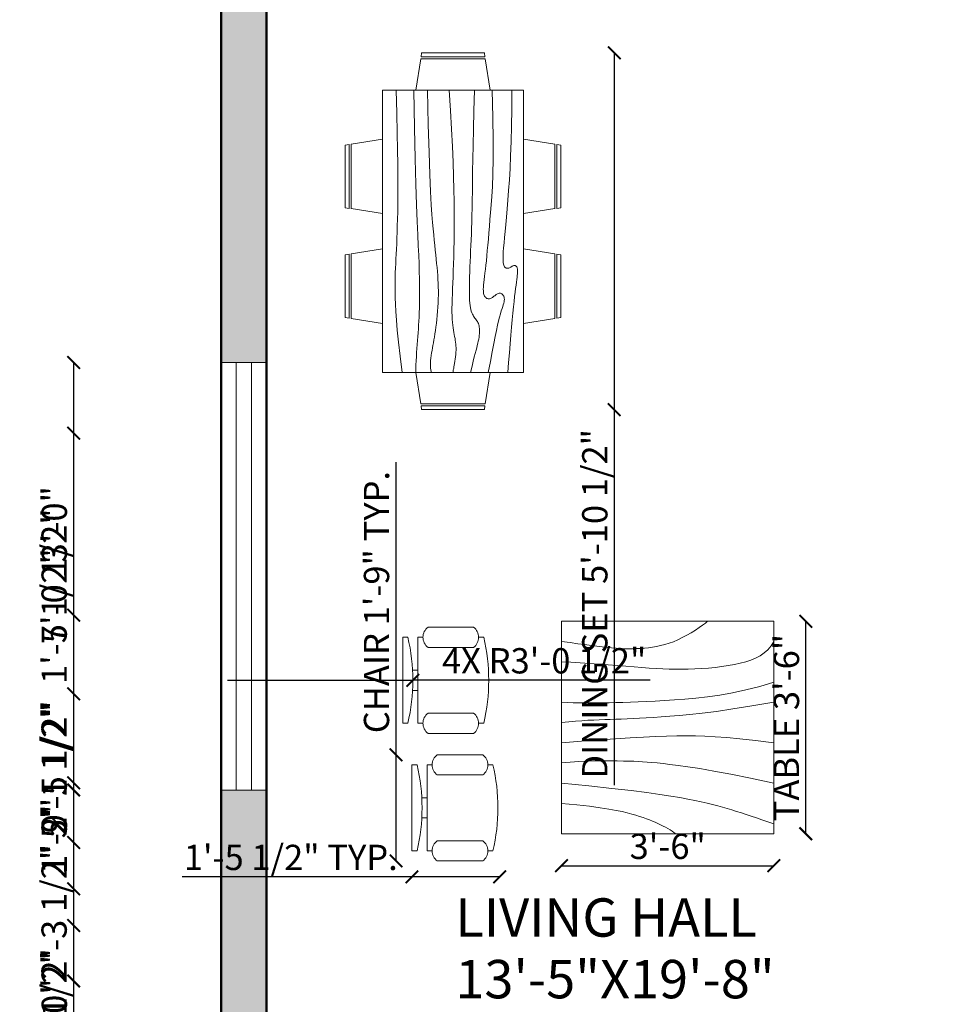
# Model space of a CAD drawing. Units: inches. Extents: x 1799 to 2247, y 1296 to 1881.
# Tile 2 of 4: x 1799 to 1983, y 1492 to 1687. Entities that reach past the tile are written whole.
import ezdxf

# ---------------------------------------------------------------- set-up
doc = ezdxf.new("R2010")
doc.units = ezdxf.units.IN
for name, color, linetype, lineweight in [('A-ANNO-DIMS', 2, 'Continuous', 18), ('A-AREA-IDEN', 7, 'Continuous', 25), ('A-FURN', 8, 'Continuous', 18), ('A-WALL', 7, 'Continuous', 50), ('window', 4, 'Continuous', 18)]:
    doc.layers.add(name, color=color, linetype=linetype, lineweight=lineweight)
doc.layers.add('A-WALL-PATT', color=18, linetype='Continuous', lineweight=13, true_color=0x000000)
doc.styles.get("Standard").update_dxf_attribs({"font": 'arial.ttf'})
doc.dimstyles.new('ISO-25', dxfattribs={"dimtxt": 5, "dimasz": 2.5, "dimexe": 1.25, "dimexo": 0.625, "dimtad": 1, "dimdec": 0, "dimlunit": 4, "dimtxsty": 'Standard', "dimblk": 'ARCHTICK', "dimcen": 2.5, "dimse1": 1, "dimse2": 1, "dimclrd": 1, "dimadec": 0, "dimazin": 0, "dimtfac": 1, "dimtdec": 0, "dimtmove": 0, "dimatfit": 3, "dimfxl": 1, "dimarcsym": 0})

# ---------------------------------------------------------------- blocks, each defined once
blk = doc.blocks.new('Dining Set - 36 x 72 in.')
for p, q in [((-22.2343, 26.00059), (-23.4847, 17.99762)), ((-22.2304, 26), (-5.7608, 26)), ((-22, 27.5), (-22.1562, 26.50042)), ((-5.8416, 26.5), (-22.1534, 26.5)), ((-22, 27.5), (-6, 27.5)), ((-5.8437, 26.49966), (-6, 27.5)), ((-4.5152, 17.99762), (-5.7655, 25.99926)), ((5.7657, 26.00059), (4.5153, 17.99762)), ((5.7696, 26), (22.2392, 26)), ((6, 27.5), (5.8438, 26.50042)), ((22.1584, 26.5), (5.8466, 26.5)), ((6, 27.5), (22, 27.5)), ((22.1563, 26.49966), (22, 27.5)), ((23.4848, 17.99762), (22.2345, 25.99926)), ((36, 18), (-36, 18)), ((-36, 18), (-36, -18)), ((36, -18), (36, 18)), ((-45.5, 8), (-44.5004, 8.15617)), ((-45.5, 8), (-45.5, -8)), ((-44.5, -8.15843), (-44.5, 8.15338)), ((-44.0006, 8.23428), (-35.9976, 9.48474)), ((-44, 8.23041), (-44, -8.23915)), ((44.0006, 8.23428), (35.9976, 9.48474)), ((44, 8.23041), (44, -8.23915)), ((44.5, -8.15843), (44.5, 8.15338)), ((45.5, 8), (44.5005, 8.15617)), ((45.5, 8), (45.5, -8)), ((-44.4997, -8.15631), (-45.5, -8)), ((-35.9976, -9.48476), (-43.9993, -8.2345)), ((35.9976, -9.48476), (43.9993, -8.2345)), ((44.4997, -8.15631), (45.5, -8)), ((-36, -18), (36, -18)), ((-22.2343, -26.0006), (-23.4847, -17.99762)), ((-4.5152, -17.99762), (-5.7655, -25.99928)), ((5.7657, -26.0006), (4.5153, -17.99762)), ((23.4848, -17.99762), (22.2345, -25.99928)), ((-22.2304, -26), (-5.7608, -26)), ((-22, -27.5), (-22.1562, -26.50044)), ((-5.8416, -26.5), (-22.1534, -26.5)), ((-22, -27.5), (-6, -27.5)), ((-5.8437, -26.49967), (-6, -27.5)), ((5.7696, -26), (22.2392, -26)), ((6, -27.5), (5.8438, -26.50044)), ((22.1584, -26.5), (5.8466, -26.5)), ((6, -27.5), (22, -27.5)), ((22.1563, -26.49967), (22, -27.5))]:
    blk.add_line(p, q)
for points in [[(-36, 15), (-31.1772, 14.97754), (-26.8079, 14.91406), (-22.8538, 14.81543), (-19.276, 14.6875), (-16.0362, 14.53613), (-13.0957, 14.36718), (-10.4159, 14.18652), (-7.9583, 14), (-5.6904, 13.81315), (-3.6035, 13.63021), (-1.6954, 13.45508), (0.0365, 13.29166), (1.5945, 13.14388), (2.9811, 13.01562), (4.1988, 12.9108), (5.25, 12.83333), (6.1393, 12.78613), (6.8802, 12.76823), (7.4883, 12.77767), (7.9792, 12.8125), (8.3685, 12.87077), (8.6719, 12.95052), (8.9049, 13.0498), (9.0833, 13.16666), (9.2205, 13.29899), (9.3216, 13.44401), (9.3895, 13.59879), (9.4271, 13.76041), (9.4373, 13.92594), (9.4232, 14.09245), (9.3875, 14.257), (9.3333, 14.41666), (9.2638, 14.56917), (9.1836, 14.71484), (9.0975, 14.85465), (9.0104, 14.98958), (8.9272, 15.1206), (8.8529, 15.2487), (8.7922, 15.37483), (8.75, 15.5), (8.7305, 15.62467), (8.7344, 15.74739), (8.7617, 15.86621), (8.8125, 15.97916), (8.8867, 16.08431), (8.9844, 16.17968), (9.1055, 16.26334), (9.25, 16.33333), (9.4189, 16.38802), (9.6172, 16.42708), (9.8506, 16.45052), (10.125, 16.45833), (10.4463, 16.45052), (10.8203, 16.42708), (11.2529, 16.38802), (11.75, 16.33333), (12.3184, 16.26318), (12.9694, 16.17838), (13.7151, 16.07991), (14.5677, 15.96875), (15.5395, 15.84586), (16.6426, 15.71224), (17.8893, 15.56884), (19.2917, 15.41666), (20.859, 15.25667), (22.5879, 15.08984), (24.4721, 14.91715), (26.5052, 14.73958), (28.6809, 14.5581), (30.9929, 14.3737), (33.4347, 14.18733), (36, 14)], [(-36, 10), (-28.9766, 10.14274), (-23.1725, 10.20442), (-18.4241, 10.19775), (-14.5677, 10.13541), (-11.4399, 10.03011), (-8.877, 9.89453), (-6.7154, 9.74137), (-4.7917, 9.58333), (-2.9698, 9.43082), (-1.2246, 9.28515), (0.4415, 9.14534), (2.026, 9.01041), (3.5266, 8.87939), (4.9408, 8.7513), (6.266, 8.62516), (7.5, 8.5), (8.6411, 8.37549), (9.6914, 8.2539), (10.6538, 8.13818), (11.5312, 8.03125), (12.3267, 7.93603), (13.043, 7.85547), (13.6831, 7.79248), (14.25, 7.75), (14.7471, 7.7303), (15.1797, 7.73307), (15.5537, 7.75732), (15.875, 7.80208), (16.1494, 7.86637), (16.3828, 7.94922), (16.5811, 8.04964), (16.75, 8.16666), (16.8944, 8.29915), (17.0143, 8.44531), (17.1089, 8.60319), (17.1771, 8.77083), (17.218, 8.94629), (17.2305, 9.1276), (17.2137, 9.31282), (17.1667, 9.5), (17.0895, 9.6875), (16.987, 9.875), (16.8649, 10.0625), (16.7292, 10.25), (16.5856, 10.4375), (16.4401, 10.625), (16.2985, 10.8125), (16.1667, 11), (16.05, 11.18733), (15.9518, 11.3737), (15.8752, 11.5581), (15.8229, 11.73958), (15.798, 11.91715), (15.8034, 12.08984), (15.842, 12.25667), (15.9167, 12.41666), (16.0295, 12.56836), (16.1784, 12.70833), (16.3605, 12.83268), (16.5729, 12.9375), (16.8127, 13.01888), (17.0768, 13.07291), (17.3625, 13.0957), (17.6667, 13.08333), (17.9894, 13.03312), (18.3418, 12.94726), (18.7382, 12.82918), (19.1927, 12.68229), (19.7195, 12.51001), (20.3327, 12.31575), (21.0465, 12.10294), (21.875, 11.875), (22.8357, 11.63354), (23.959, 11.37304), (25.2786, 11.08618), (26.8282, 10.76562), (28.6414, 10.40405), (30.752, 9.99414), (33.1936, 9.52856), (36, 9)], [(-36, 5.5), (-30.7157, 5.3348), (-26.069, 5.20963), (-21.9946, 5.11767), (-18.4271, 5.05208), (-15.3009, 5.00602), (-12.5508, 4.97265), (-10.1112, 4.94515), (-7.9167, 4.91666), (-5.909, 4.88167), (-4.0586, 4.83984), (-2.3429, 4.79215), (-0.7396, 4.73958), (0.7739, 4.6831), (2.22, 4.6237), (3.6213, 4.56233), (5, 4.5), (6.373, 4.43782), (7.7344, 4.3776), (9.0723, 4.32129), (10.375, 4.27083), (11.6309, 4.22819), (12.8281, 4.19531), (13.9551, 4.17415), (15, 4.16666), (15.954, 4.17448), (16.819, 4.19791), (17.6001, 4.23698), (18.3021, 4.29166), (18.9299, 4.36198), (19.4883, 4.44791), (19.9823, 4.54948), (20.4167, 4.66666), (20.7969, 4.79899), (21.1302, 4.94401), (21.4245, 5.09879), (21.6875, 5.26041), (21.9271, 5.42594), (22.1511, 5.59245), (22.3672, 5.757), (22.5834, 5.91666), (22.8065, 6.06868), (23.0404, 6.21093), (23.2879, 6.34147), (23.5521, 6.45833), (23.8358, 6.55957), (24.142, 6.64323), (24.4735, 6.70735), (24.8334, 6.75), (25.2235, 6.76969), (25.642, 6.76692), (26.0858, 6.74267), (26.5521, 6.69791), (27.0379, 6.63362), (27.5404, 6.55078), (28.0565, 6.45036), (28.5834, 6.33333), (29.1242, 6.19987), (29.7071, 6.04687), (30.3661, 5.87044), (31.1354, 5.66666), (32.0493, 5.43164), (33.142, 5.16146), (34.4475, 4.85221), (36, 4.5)], [(-36, -1), (-30.7915, -0.6591), (-26.0195, -0.38216), (-21.6519, -0.16284), (-17.6563, 0.00521), (-14.0005, 0.12833), (-10.6523, 0.21289), (-7.5796, 0.26522), (-4.75, 0.29166), (-2.134, 0.29793), (0.2878, 0.28711), (2.5317, 0.26163), (4.6146, 0.22396), (6.5529, 0.17651), (8.3633, 0.12174), (10.0623, 0.06209), (11.6667, 0), (13.1899, -0.06201), (14.6341, -0.1211), (15.9982, -0.17432), (17.2813, -0.21875), (18.4823, -0.25147), (19.6003, -0.26953), (20.6343, -0.27002), (21.5834, -0.25), (22.4481, -0.20768), (23.2357, -0.14584), (23.9549, -0.06836), (24.6146, 0.02083), (25.2235, 0.11784), (25.7904, 0.21875), (26.3241, 0.31966), (26.8334, 0.41666), (27.3265, 0.50618), (27.8099, 0.58593), (28.2894, 0.65397), (28.7709, 0.70833), (29.2601, 0.74707), (29.763, 0.76823), (30.2855, 0.76985), (30.8334, 0.75), (31.4088, 0.70784), (31.9994, 0.64713), (32.589, 0.57275), (33.1615, 0.48958), (33.7008, 0.4025), (34.1908, 0.3164), (34.6153, 0.23616), (34.9584, 0.16666), (35.2099, 0.11165), (35.3848, 0.07031), (35.504, 0.04069), (35.5886, 0.02083), (35.6594, 0.00879), (35.7377, 0.0026), (35.8442, 0.00032), (36, 0)], [(-36, -6.5), (-27.1843, -6.31267), (-20.084, -6.1263), (-14.469, -5.9419), (-10.1094, -5.76042), (-6.7752, -5.58285), (-4.2363, -5.41016), (-2.2629, -5.24333), (-0.625, -5.08334), (0.8708, -4.93099), (2.2715, -4.78646), (3.5872, -4.64974), (4.8281, -4.52084), (6.0046, -4.39974), (7.127, -4.28646), (8.2053, -4.18099), (9.25, -4.08334), (10.2705, -3.99382), (11.2734, -3.91407), (12.2647, -3.84603), (13.25, -3.79167), (14.2354, -3.75293), (15.2266, -3.73177), (16.2295, -3.73015), (17.25, -3.75), (18.2912, -3.79248), (19.3451, -3.85547), (20.4009, -3.93604), (21.4479, -4.03125), (22.4754, -4.13819), (23.4727, -4.25391), (24.4289, -4.37549), (25.3334, -4.5), (26.1785, -4.62492), (26.9694, -4.74935), (27.7145, -4.87281), (28.4219, -4.99479), (29.1, -5.11483), (29.7572, -5.23242), (30.4016, -5.34709), (31.0417, -5.45834), (31.6837, -5.56437), (32.3262, -5.65821), (32.9658, -5.73153), (33.599, -5.77604), (34.2224, -5.78345), (34.8327, -5.74545), (35.4264, -5.65373), (36, -5.5)], [(-36, -10), (-26.4022, -9.81299), (-18.4675, -9.62891), (-11.9839, -9.45069), (-6.7396, -9.28125), (-2.5226, -9.12354), (0.8789, -8.98047), (3.6769, -8.85498), (6.0833, -8.75), (8.2767, -8.66765), (10.3021, -8.60677), (12.1712, -8.56543), (13.8958, -8.54167), (15.4876, -8.53353), (16.9583, -8.53907), (18.3197, -8.55632), (19.5834, -8.58334), (20.7616, -8.61841), (21.8685, -8.66081), (22.9188, -8.71004), (23.9271, -8.76563), (24.9081, -8.82707), (25.8763, -8.89388), (26.8465, -8.96558), (27.8334, -9.04167), (28.8474, -9.12118), (29.8828, -9.20117), (30.93, -9.27824), (31.9792, -9.34896), (33.0205, -9.40991), (34.0443, -9.45768), (35.0407, -9.48885), (36, -9.5)], [(-36, -14.5), (-30.0881, -14.33513), (-25.0332, -14.21224), (-20.7312, -14.12647), (-17.0781, -14.07292), (-13.97, -14.04671), (-11.3027, -14.04297), (-8.9724, -14.05681), (-6.875, -14.08334), (-4.9224, -14.11833), (-3.0905, -14.16016), (-1.3709, -14.20785), (0.2448, -14.26042), (1.7647, -14.3169), (3.1973, -14.3763), (4.5507, -14.43767), (5.8333, -14.5), (7.0554, -14.5621), (8.235, -14.62175), (9.3922, -14.67652), (10.5469, -14.72396), (11.7192, -14.76164), (12.929, -14.78711), (14.1965, -14.79794), (15.5417, -14.79167), (16.9933, -14.76424), (18.6152, -14.70508), (20.4804, -14.60197), (22.6615, -14.44271), (25.2312, -14.21509), (28.2624, -13.9069), (31.8277, -13.50594), (36, -13)]]:
    blk.add_lwpolyline(points)
blk = doc.blocks.new('Table - Square Woodgrain 42 x 42 in.')
blk.add_line((0, -42), (42, -42))
for points in [[(0, -4), (1.704, -4.2172), (3.2358, -4.4188), (4.615, -4.604), (5.8615, -4.7721), (6.9951, -4.9224), (8.0357, -5.0541), (9.0031, -5.1667), (9.9171, -5.2594), (10.7951, -5.3316), (11.6445, -5.3836), (12.4702, -5.4157), (13.277, -5.4283), (14.0698, -5.4217), (14.8535, -5.3964), (15.6331, -5.3526), (16.4133, -5.2908), (17.1986, -5.2103), (17.9913, -5.1062), (18.793, -4.9727), (19.6056, -4.8038), (20.4307, -4.5937), (21.2701, -4.3365), (22.1256, -4.0262), (22.9989, -3.6571), (23.888, -3.2272), (24.7756, -2.7516), (25.6408, -2.2491), (26.4624, -1.7387), (27.2195, -1.2395), (27.891, -0.7703), (28.456, -0.3501), (28.8934, 0.002)], [(0, -42), (0, 0), (42, 0), (42, -42)], [(0, -8), (1.8203, -8.1001), (3.6741, -8.2149), (5.5411, -8.3408), (7.4011, -8.4741), (9.2339, -8.6112), (11.0193, -8.7484), (12.7371, -8.8821), (14.3671, -9.0086), (15.8954, -9.1246), (17.3337, -9.2278), (18.6997, -9.3159), (20.0116, -9.387), (21.2871, -9.4389), (22.5442, -9.4696), (23.8008, -9.477), (25.0749, -9.459), (26.3791, -9.4137), (27.7049, -9.3403), (29.0383, -9.2382), (30.3655, -9.1068), (31.6728, -8.9455), (32.9461, -8.7535), (34.1717, -8.5304), (35.3358, -8.2756), (36.4268, -7.9863), (37.443, -7.6521), (38.3849, -7.2603), (39.253, -6.7986), (40.048, -6.2542), (40.7705, -5.6147), (41.421, -4.8674), (42, -4)], [(42, -12), (39.1784, -12.8621), (36.4519, -13.5654), (33.8246, -14.1294), (31.3004, -14.5731), (28.8832, -14.9161), (26.577, -15.1775), (24.3858, -15.3768), (22.3136, -15.5332), (20.3622, -15.6632), (18.5254, -15.7718), (16.7947, -15.8612), (15.1618, -15.9338), (13.6183, -15.9916), (12.1558, -16.0369), (10.7659, -16.0718), (9.4403, -16.0987), (8.1703, -16.1191), (6.9461, -16.1325), (5.7577, -16.1377), (4.595, -16.1335), (3.4479, -16.1188), (2.3064, -16.0924), (1.1604, -16.0532), (0, -16)], [(42, -16), (37.6529, -16.7365), (33.8802, -17.329), (30.6179, -17.7961), (27.8015, -18.1561), (25.3668, -18.4275), (23.2497, -18.6288), (21.3859, -18.7785), (19.7111, -18.8949), (18.1693, -18.9939), (16.7375, -19.0795), (15.401, -19.1534), (14.1449, -19.217), (12.9544, -19.2717), (11.8148, -19.3191), (10.7113, -19.3606), (9.6291, -19.3976), (8.5534, -19.4323), (7.47, -19.4689), (6.3643, -19.5122), (5.222, -19.5672), (4.0288, -19.6386), (2.7703, -19.7313), (1.4321, -19.8501), (0, -20)], [(0, -24), (3.9243, -23.6805), (7.4766, -23.4138), (10.6891, -23.1954), (13.5943, -23.0205), (16.2247, -22.8847), (18.6125, -22.7832), (20.7903, -22.7116), (22.7903, -22.6651), (24.6563, -22.642), (26.4764, -22.6507), (28.35, -22.7024), (30.3766, -22.8084), (32.6555, -22.98), (35.2861, -23.2283), (38.3678, -23.5645), (42, -24)], [(42, -32), (37.392, -31.017), (33.4585, -30.2231), (30.1291, -29.5949), (27.3334, -29.109), (25.0009, -28.742), (23.0612, -28.4707), (21.4439, -28.2716), (20.0786, -28.1215), (18.8998, -28.0002), (17.8609, -27.9014), (16.9206, -27.8219), (16.0371, -27.7588), (15.1691, -27.709), (14.2748, -27.6693), (13.3128, -27.6368), (12.2415, -27.6083), (11.0295, -27.5824), (9.6867, -27.5643), (8.233, -27.5608), (6.6884, -27.5787), (5.0728, -27.6248), (3.4062, -27.7058), (1.7086, -27.8286), (0, -28)], [(0, -32), (5.4026, -32.5358), (9.9494, -33.019), (13.7424, -33.4553), (16.8834, -33.8505), (19.4743, -34.2106), (21.6171, -34.5413), (23.4136, -34.8486), (24.9657, -35.1382), (26.3614, -35.4156), (27.6332, -35.6841), (28.7995, -35.9467), (29.8788, -36.2064), (30.8897, -36.4661), (31.8507, -36.7288), (32.7802, -36.9973), (33.6968, -37.2747), (34.6175, -37.5635), (35.5531, -37.8651), (36.5128, -38.1805), (37.506, -38.5108), (38.5421, -38.8568), (39.6302, -39.2197), (40.7797, -39.6004), (42, -40)], [(0, -36), (3.0098, -36.2857), (5.5354, -36.5643), (7.6368, -36.8359), (9.374, -37.1009), (10.807, -37.3597), (11.9957, -37.6126), (13.0002, -37.8599), (13.8804, -38.102), (14.6874, -38.3393), (15.4365, -38.5729), (16.1338, -38.8041), (16.7858, -39.0341), (17.3987, -39.264), (17.9787, -39.4952), (18.5322, -39.7288), (19.0655, -39.9662), (19.5832, -40.2081), (20.0842, -40.4544), (20.5657, -40.7046), (21.0249, -40.9581), (21.459, -41.2144), (21.8653, -41.4731), (22.2409, -41.7335), (22.5831, -41.9951)]]:
    blk.add_lwpolyline(points)
blk = doc.blocks.new('Chair - Desk')
for p, q in [((-8.5, 0), (-8.5, -1)), ((-8.5, 0), (8.5, 0)), ((8.5, 0), (8.5, -1)), ((-2, -3), (-2, -1.9355)), ((-8.5, -3), (-8.5, -4)), ((-8.5, -3), (8.5, -3)), ((2, -1.9576), (2, -3)), ((8.5, -3), (8.5, -4)), ((-10.5, -5), (-10.5, -14)), ((-6.5, -14), (-6.5, -5)), ((6.5, -5), (6.5, -14)), ((10.5, -14), (10.5, -5)), ((-8.5, -15), (-8.5, -16)), ((8.5, -15), (8.5, -16))]:
    blk.add_line(p, q)
for centre, radius, start, end in [((0, 34.625), 36.625, 256.5803, 283.4197), ((-8.5, -6.5), 2.5, 36.8699, 143.1301), ((8.5, -6.5), 2.5, 36.8699, 143.1301), ((-8.5, -12.5), 2.5, 216.8699, 323.1301), ((8.5, -12.5), 2.5, 216.8699, 323.1301), ((0, 19.625), 36.625, 256.5803, 283.4197)]:
    blk.add_arc(centre, radius, start, end)
blk = doc.blocks.new('_ArchTick')
at = {"color": 0, "linetype": 'ByBlock', "const_width": 0.15}
blk.add_lwpolyline([(-0.5, -0.5), (0.5, 0.5)], dxfattribs=at)
blk = doc.blocks.new('*D18')
at = {"layer": 'A-ANNO-DIMS', "color": 1, "lineweight": -2, "transparency": 16777216}
for p, q in [((1873.03, 1541.28), (1873.03, 1599.13)), ((1873.03, 1520.28), (1873.03, 1541.28))]:
    blk.add_line(p, q, dxfattribs=at)
at = {"layer": 'Defpoints', "color": 0, "transparency": 16777216}
for p in [(1873.03, 1541.28), (1876.18, 1541.28), (1876.18, 1520.28)]:
    blk.add_point(p, dxfattribs=at)
at = {"layer": 'A-ANNO-DIMS', "color": 1, "lineweight": -2, "transparency": 16777216, "xscale": 2.5, "yscale": 2.5, "zscale": 2.5}
for p, rotation in [((1873.03, 1541.28), 90), ((1873.03, 1520.28), 270)]:
    blk.add_blockref('_ArchTick', p, dxfattribs=dict(at, rotation=rotation))
at = {"layer": 'A-ANNO-DIMS', "color": 0, "transparency": 16777216, "insert": (1869.82, 1571.45), "char_height": 5, "attachment_point": 5, "rotation": 90}
blk.add_mtext('CHAIR 1\'-9" TYP.', dxfattribs=at)
blk = doc.blocks.new('*D19')
at = {"layer": 'A-ANNO-DIMS', "color": 1, "lineweight": -2, "transparency": 16777216}
for p, q in [((1876.18, 1517.13), (1830.78, 1517.13)), ((1893.52, 1517.13), (1876.18, 1517.13))]:
    blk.add_line(p, q, dxfattribs=at)
at = {"layer": 'Defpoints', "color": 0, "transparency": 16777216}
for p in [(1876.18, 1520.28), (1893.52, 1520.28), (1876.18, 1517.13)]:
    blk.add_point(p, dxfattribs=at)
at = {"layer": 'A-ANNO-DIMS', "color": 1, "lineweight": -2, "transparency": 16777216, "xscale": 2.5, "yscale": 2.5, "zscale": 2.5, "rotation": 180}
blk.add_blockref('_ArchTick', (1876.18, 1517.13), dxfattribs=at)
at = {"layer": 'A-ANNO-DIMS', "color": 1, "lineweight": -2, "transparency": 16777216, "xscale": 2.5, "yscale": 2.5, "zscale": 2.5}
blk.add_blockref('_ArchTick', (1893.52, 1517.13), dxfattribs=at)
at = {"layer": 'A-ANNO-DIMS', "color": 0, "transparency": 16777216, "insert": (1852.23, 1520.34), "char_height": 5, "attachment_point": 5}
blk.add_mtext('1\'-5 1/2" TYP.', dxfattribs=at)
blk = doc.blocks.new('*D22')
at = {"layer": 'A-ANNO-DIMS', "color": 1, "lineweight": -2, "transparency": 16777216}
for p, q in [((1916.18, 1680), (1916.18, 1609.48)), ((1916.18, 1609.48), (1916.18, 1535.24))]:
    blk.add_line(p, q, dxfattribs=at)
at = {"layer": 'Defpoints', "color": 0, "transparency": 16777216}
for p in [(1905.61, 1680), (1905.61, 1609.48), (1916.18, 1609.48)]:
    blk.add_point(p, dxfattribs=at)
at = {"layer": 'A-ANNO-DIMS', "color": 1, "lineweight": -2, "transparency": 16777216, "xscale": 2.5, "yscale": 2.5, "zscale": 2.5}
for p, rotation in [((1916.18, 1680), 90), ((1916.18, 1609.48), 270)]:
    blk.add_blockref('_ArchTick', p, dxfattribs=dict(at, rotation=rotation))
at = {"layer": 'A-ANNO-DIMS', "color": 0, "transparency": 16777216, "insert": (1912.97, 1571.11), "char_height": 5, "attachment_point": 5, "rotation": 90}
blk.add_mtext('DINING SET 5\'-10 1/2"', dxfattribs=at)
blk = doc.blocks.new('*D23')
at = {"layer": 'A-ANNO-DIMS', "color": 1, "lineweight": -2, "transparency": 16777216}
blk.add_line((1862.99, 1690.58), (1905.61, 1690.58), dxfattribs=at)
at = {"layer": 'Defpoints', "color": 0, "transparency": 16777216}
for p in [(1905.61, 1690.58), (1862.99, 1680), (1905.61, 1680)]:
    blk.add_point(p, dxfattribs=at)
at = {"layer": 'A-ANNO-DIMS', "color": 1, "lineweight": -2, "transparency": 16777216, "xscale": 2.5, "yscale": 2.5, "zscale": 2.5, "rotation": 180}
blk.add_blockref('_ArchTick', (1862.99, 1690.58), dxfattribs=at)
at = {"layer": 'A-ANNO-DIMS', "color": 1, "lineweight": -2, "transparency": 16777216, "xscale": 2.5, "yscale": 2.5, "zscale": 2.5}
blk.add_blockref('_ArchTick', (1905.61, 1690.58), dxfattribs=at)
at = {"layer": 'A-ANNO-DIMS', "color": 0, "transparency": 16777216, "insert": (1884.3, 1693.79), "char_height": 5, "attachment_point": 5}
blk.add_mtext('3\'-6 1/2"', dxfattribs=at)
blk = doc.blocks.new('*D30')
at = {"layer": 'A-ANNO-DIMS', "color": 1, "lineweight": -2, "transparency": 16777216}
blk.add_line((1954.04, 1525.65), (1954.04, 1567.65), dxfattribs=at)
at = {"layer": 'Defpoints', "color": 0, "transparency": 16777216}
for p in [(1947.74, 1567.65), (1954.04, 1567.65), (1947.74, 1525.65)]:
    blk.add_point(p, dxfattribs=at)
at = {"layer": 'A-ANNO-DIMS', "color": 1, "lineweight": -2, "transparency": 16777216, "xscale": 2.5, "yscale": 2.5, "zscale": 2.5}
for p, rotation in [((1954.04, 1567.65), 90), ((1954.04, 1525.65), 270)]:
    blk.add_blockref('_ArchTick', p, dxfattribs=dict(at, rotation=rotation))
at = {"layer": 'A-ANNO-DIMS', "color": 0, "transparency": 16777216, "insert": (1950.86, 1546.65), "char_height": 5, "attachment_point": 5, "rotation": 90}
blk.add_mtext('TABLE 3\'-6"', dxfattribs=at)
blk = doc.blocks.new('*D31')
at = {"layer": 'A-ANNO-DIMS', "color": 1, "lineweight": -2, "transparency": 16777216}
blk.add_line((1905.74, 1519.35), (1947.74, 1519.35), dxfattribs=at)
at = {"layer": 'Defpoints', "color": 0, "transparency": 16777216}
for p in [(1905.74, 1525.65), (1947.74, 1525.65), (1947.74, 1519.35)]:
    blk.add_point(p, dxfattribs=at)
at = {"layer": 'A-ANNO-DIMS', "color": 1, "lineweight": -2, "transparency": 16777216, "xscale": 2.5, "yscale": 2.5, "zscale": 2.5, "rotation": 180}
blk.add_blockref('_ArchTick', (1905.74, 1519.35), dxfattribs=at)
at = {"layer": 'A-ANNO-DIMS', "color": 1, "lineweight": -2, "transparency": 16777216, "xscale": 2.5, "yscale": 2.5, "zscale": 2.5}
blk.add_blockref('_ArchTick', (1947.74, 1519.35), dxfattribs=at)
at = {"layer": 'A-ANNO-DIMS', "color": 0, "transparency": 16777216, "insert": (1926.74, 1522.53), "char_height": 5, "attachment_point": 5}
blk.add_mtext('3\'-6"', dxfattribs=at)
blk = doc.blocks.new('*D35')
at = {"layer": 'A-ANNO-DIMS', "color": 1, "lineweight": -2, "transparency": 16777216}
blk.add_line((1960.46, 1297.17), (2076.46, 1297.17), dxfattribs=at)
at = {"layer": 'Defpoints', "color": 0, "transparency": 16777216}
for p in [(1960.46, 1821.32), (2076.46, 1821.32), (2076.46, 1297.17)]:
    blk.add_point(p, dxfattribs=at)
at = {"layer": 'A-ANNO-DIMS', "color": 1, "lineweight": -2, "transparency": 16777216, "xscale": 2.5, "yscale": 2.5, "zscale": 2.5, "rotation": 180}
blk.add_blockref('_ArchTick', (1960.46, 1297.17), dxfattribs=at)
at = {"layer": 'A-ANNO-DIMS', "color": 1, "lineweight": -2, "transparency": 16777216, "xscale": 2.5, "yscale": 2.5, "zscale": 2.5}
blk.add_blockref('_ArchTick', (2076.46, 1297.17), dxfattribs=at)
at = {"layer": 'A-ANNO-DIMS', "color": 0, "transparency": 16777216, "insert": (2018.46, 1300.35), "char_height": 5, "attachment_point": 5}
blk.add_mtext('9\'-8"', dxfattribs=at)
blk = doc.blocks.new('*D47')
at = {"layer": 'A-ANNO-DIMS', "color": 1, "lineweight": -2, "transparency": 16777216}
blk.add_line((1914.89, 1297.17), (1950.83, 1297.17), dxfattribs=at)
at = {"layer": 'Defpoints', "color": 0, "transparency": 16777216}
for p in [(1914.89, 1701.32), (1950.83, 1701.32), (1950.83, 1297.17)]:
    blk.add_point(p, dxfattribs=at)
at = {"layer": 'A-ANNO-DIMS', "color": 1, "lineweight": -2, "transparency": 16777216, "xscale": 2.5, "yscale": 2.5, "zscale": 2.5, "rotation": 180}
blk.add_blockref('_ArchTick', (1914.89, 1297.17), dxfattribs=at)
at = {"layer": 'A-ANNO-DIMS', "color": 1, "lineweight": -2, "transparency": 16777216, "xscale": 2.5, "yscale": 2.5, "zscale": 2.5}
blk.add_blockref('_ArchTick', (1950.83, 1297.17), dxfattribs=at)
at = {"layer": 'A-ANNO-DIMS', "color": 0, "transparency": 16777216, "insert": (1932.86, 1300.35), "char_height": 5, "attachment_point": 5}
blk.add_mtext('3\'-0"', dxfattribs=at)
blk = doc.blocks.new('*D48')
at = {"layer": 'A-ANNO-DIMS', "color": 1, "lineweight": -2, "transparency": 16777216}
blk.add_line((1962.42, 1859.47), (1998.36, 1859.47), dxfattribs=at)
at = {"layer": 'Defpoints', "color": 0, "transparency": 16777216}
for p in [(1998.36, 1859.47), (1962.42, 1353.51), (1998.36, 1353.51)]:
    blk.add_point(p, dxfattribs=at)
at = {"layer": 'A-ANNO-DIMS', "color": 1, "lineweight": -2, "transparency": 16777216, "xscale": 2.5, "yscale": 2.5, "zscale": 2.5, "rotation": 180}
blk.add_blockref('_ArchTick', (1962.42, 1859.47), dxfattribs=at)
at = {"layer": 'A-ANNO-DIMS', "color": 1, "lineweight": -2, "transparency": 16777216, "xscale": 2.5, "yscale": 2.5, "zscale": 2.5}
blk.add_blockref('_ArchTick', (1998.36, 1859.47), dxfattribs=at)
at = {"layer": 'A-ANNO-DIMS', "color": 0, "transparency": 16777216, "insert": (1980.39, 1862.65), "char_height": 5, "attachment_point": 5}
blk.add_mtext('3\'-0"', dxfattribs=at)
blk = doc.blocks.new('*D49')
at = {"layer": 'A-ANNO-DIMS', "color": 1, "lineweight": -2, "transparency": 16777216}
blk.add_line((1809.31, 1534.31), (1809.31, 1618.8), dxfattribs=at)
at = {"layer": 'Defpoints', "color": 0, "transparency": 16777216}
for p in [(1809.31, 1618.8), (1838.46, 1618.8), (1838.46, 1534.31)]:
    blk.add_point(p, dxfattribs=at)
at = {"layer": 'A-ANNO-DIMS', "color": 1, "lineweight": -2, "transparency": 16777216, "xscale": 2.5, "yscale": 2.5, "zscale": 2.5}
for p, rotation in [((1809.31, 1618.8), 90), ((1809.31, 1534.31), 270)]:
    blk.add_blockref('_ArchTick', p, dxfattribs=dict(at, rotation=rotation))
at = {"layer": 'A-ANNO-DIMS', "color": 0, "transparency": 16777216, "insert": (1806.1, 1576.56), "char_height": 5, "attachment_point": 5, "rotation": 90}
blk.add_mtext('7\'-0 1/2"', dxfattribs=at)
blk = doc.blocks.new('*D50')
at = {"layer": 'A-ANNO-DIMS', "color": 1, "lineweight": -2, "transparency": 16777216}
blk.add_line((1809.31, 1444.97), (1809.31, 1534.31), dxfattribs=at)
at = {"layer": 'Defpoints', "color": 0, "transparency": 16777216}
for p in [(1809.31, 1534.31), (1838.46, 1534.31), (1838.46, 1444.97)]:
    blk.add_point(p, dxfattribs=at)
at = {"layer": 'A-ANNO-DIMS', "color": 1, "lineweight": -2, "transparency": 16777216, "xscale": 2.5, "yscale": 2.5, "zscale": 2.5}
for p, rotation in [((1809.31, 1534.31), 90), ((1809.31, 1444.97), 270)]:
    blk.add_blockref('_ArchTick', p, dxfattribs=dict(at, rotation=rotation))
at = {"layer": 'A-ANNO-DIMS', "color": 0, "transparency": 16777216, "insert": (1806.1, 1489.64), "char_height": 5, "attachment_point": 5, "rotation": 90}
blk.add_mtext('7\'-5 1/2"', dxfattribs=at)
blk = doc.blocks.new('*D57')
at = {"layer": 'A-ANNO-DIMS', "color": 1, "lineweight": -2, "transparency": 16777216}
blk.add_line((1875.53, 1297.17), (1901.39, 1297.17), dxfattribs=at)
at = {"layer": 'Defpoints', "color": 0, "transparency": 16777216}
for p in [(1901.39, 1801.76), (1875.53, 1797.03), (1901.39, 1297.17)]:
    blk.add_point(p, dxfattribs=at)
at = {"layer": 'A-ANNO-DIMS', "color": 1, "lineweight": -2, "transparency": 16777216, "xscale": 2.5, "yscale": 2.5, "zscale": 2.5, "rotation": 180}
blk.add_blockref('_ArchTick', (1875.53, 1297.17), dxfattribs=at)
at = {"layer": 'A-ANNO-DIMS', "color": 1, "lineweight": -2, "transparency": 16777216, "xscale": 2.5, "yscale": 2.5, "zscale": 2.5}
blk.add_blockref('_ArchTick', (1901.39, 1297.17), dxfattribs=at)
at = {"layer": 'A-ANNO-DIMS', "color": 0, "transparency": 16777216, "insert": (1888.46, 1300.3), "char_height": 5, "attachment_point": 5}
blk.add_mtext('2\'-2"', dxfattribs=at)
blk = doc.blocks.new('*D58')
at = {"layer": 'A-ANNO-DIMS', "color": 1, "lineweight": -2, "transparency": 16777216}
blk.add_line((1809.31, 1568.87), (1809.31, 1604.81), dxfattribs=at)
at = {"layer": 'Defpoints', "color": 0, "transparency": 16777216}
for p in [(1809.31, 1604.81), (2003.46, 1604.81), (2003.46, 1568.87)]:
    blk.add_point(p, dxfattribs=at)
at = {"layer": 'A-ANNO-DIMS', "color": 1, "lineweight": -2, "transparency": 16777216, "xscale": 2.5, "yscale": 2.5, "zscale": 2.5}
for p, rotation in [((1809.31, 1604.81), 90), ((1809.31, 1568.87), 270)]:
    blk.add_blockref('_ArchTick', p, dxfattribs=dict(at, rotation=rotation))
at = {"layer": 'A-ANNO-DIMS', "color": 0, "transparency": 16777216, "insert": (1806.13, 1586.84), "char_height": 5, "attachment_point": 5, "rotation": 90}
blk.add_mtext('3\'-0"', dxfattribs=at)
blk = doc.blocks.new('*D59')
at = {"layer": 'A-ANNO-DIMS', "color": 1, "lineweight": -2, "transparency": 16777216}
blk.add_line((1809.31, 1507.52), (1809.31, 1568.87), dxfattribs=at)
at = {"layer": 'Defpoints', "color": 0, "transparency": 16777216}
for p in [(1809.31, 1568.87), (2003.46, 1568.87), (2003.46, 1507.52)]:
    blk.add_point(p, dxfattribs=at)
at = {"layer": 'A-ANNO-DIMS', "color": 1, "lineweight": -2, "transparency": 16777216, "xscale": 2.5, "yscale": 2.5, "zscale": 2.5}
for p, rotation in [((1809.31, 1568.87), 90), ((1809.31, 1507.52), 270)]:
    blk.add_blockref('_ArchTick', p, dxfattribs=dict(at, rotation=rotation))
at = {"layer": 'A-ANNO-DIMS', "color": 0, "transparency": 16777216, "insert": (1806.1, 1538.19), "char_height": 5, "attachment_point": 5, "rotation": 90}
blk.add_mtext('5\'-1 1/2"', dxfattribs=at)
blk = doc.blocks.new('*D60')
at = {"layer": 'A-ANNO-DIMS', "color": 1, "lineweight": -2, "transparency": 16777216}
blk.add_line((1809.31, 1471.58), (1809.31, 1507.52), dxfattribs=at)
at = {"layer": 'Defpoints', "color": 0, "transparency": 16777216}
for p in [(1809.31, 1507.52), (2003.46, 1507.52), (2003.46, 1471.58)]:
    blk.add_point(p, dxfattribs=at)
at = {"layer": 'A-ANNO-DIMS', "color": 1, "lineweight": -2, "transparency": 16777216, "xscale": 2.5, "yscale": 2.5, "zscale": 2.5}
for p, rotation in [((1809.31, 1507.52), 90), ((1809.31, 1471.58), 270)]:
    blk.add_blockref('_ArchTick', p, dxfattribs=dict(at, rotation=rotation))
at = {"layer": 'A-ANNO-DIMS', "color": 0, "transparency": 16777216, "insert": (1806.13, 1489.55), "char_height": 5, "attachment_point": 5, "rotation": 90}
blk.add_mtext('3\'-0"', dxfattribs=at)
blk = doc.blocks.new('*D61')
at = {"layer": 'A-ANNO-DIMS', "color": 1, "lineweight": -2, "transparency": 16777216}
for p, q in [((1838.46, 1297.17), (1847.46, 1297.17)), ((1847.46, 1297.17), (1864.5, 1297.17))]:
    blk.add_line(p, q, dxfattribs=at)
at = {"layer": 'Defpoints', "color": 0, "transparency": 16777216}
for p in [(1838.46, 1830.32), (1847.46, 1821.32), (1847.46, 1297.17)]:
    blk.add_point(p, dxfattribs=at)
at = {"layer": 'A-ANNO-DIMS', "color": 1, "lineweight": -2, "transparency": 16777216, "xscale": 2.5, "yscale": 2.5, "zscale": 2.5, "rotation": 180}
blk.add_blockref('_ArchTick', (1838.46, 1297.17), dxfattribs=at)
at = {"layer": 'A-ANNO-DIMS', "color": 1, "lineweight": -2, "transparency": 16777216, "xscale": 2.5, "yscale": 2.5, "zscale": 2.5}
blk.add_blockref('_ArchTick', (1847.46, 1297.17), dxfattribs=at)
at = {"layer": 'A-ANNO-DIMS', "color": 0, "transparency": 16777216, "insert": (1857.23, 1300.35), "char_height": 5, "attachment_point": 5}
blk.add_mtext('0\'-9"', dxfattribs=at)
blk = doc.blocks.new('*D64')
at = {"layer": 'A-ANNO-DIMS', "color": 1, "lineweight": -2, "transparency": 16777216}
blk.add_line((1809.31, 1496.56), (1809.31, 1523.93), dxfattribs=at)
at = {"layer": 'Defpoints', "color": 0, "transparency": 16777216}
for p in [(1809.31, 1523.93), (2070.46, 1523.93), (2070.46, 1496.56)]:
    blk.add_point(p, dxfattribs=at)
at = {"layer": 'A-ANNO-DIMS', "color": 1, "lineweight": -2, "transparency": 16777216, "xscale": 2.5, "yscale": 2.5, "zscale": 2.5}
for p, rotation in [((1809.31, 1523.93), 90), ((1809.31, 1496.56), 270)]:
    blk.add_blockref('_ArchTick', p, dxfattribs=dict(at, rotation=rotation))
at = {"layer": 'A-ANNO-DIMS', "color": 0, "transparency": 16777216, "insert": (1806.09, 1510.25), "char_height": 5, "attachment_point": 5, "rotation": 90}
blk.add_mtext('2\'-3 1/2"', dxfattribs=at)
blk = doc.blocks.new('*D65')
at = {"layer": 'A-ANNO-DIMS', "color": 1, "lineweight": -2, "transparency": 16777216}
blk.add_line((1809.31, 1523.93), (1809.31, 1553.32), dxfattribs=at)
at = {"layer": 'Defpoints', "color": 0, "transparency": 16777216}
for p in [(1809.31, 1553.32), (2070.46, 1553.32), (2070.46, 1523.93)]:
    blk.add_point(p, dxfattribs=at)
at = {"layer": 'A-ANNO-DIMS', "color": 1, "lineweight": -2, "transparency": 16777216, "xscale": 2.5, "yscale": 2.5, "zscale": 2.5}
for p, rotation in [((1809.31, 1553.32), 90), ((1809.31, 1523.93), 270)]:
    blk.add_blockref('_ArchTick', p, dxfattribs=dict(at, rotation=rotation))
at = {"layer": 'A-ANNO-DIMS', "color": 0, "transparency": 16777216, "insert": (1806.1, 1538.62), "char_height": 5, "attachment_point": 5, "rotation": 90}
blk.add_mtext('2\'-5 1/2"', dxfattribs=at)
blk = doc.blocks.new('*D67')
at = {"layer": 'A-ANNO-DIMS', "color": 1, "lineweight": -2, "transparency": 16777216}
blk.add_line((1809.31, 1514.75), (1809.31, 1535.75), dxfattribs=at)
at = {"layer": 'Defpoints', "color": 0, "transparency": 16777216}
for p in [(1809.31, 1535.75), (2145.1, 1535.75), (2145.1, 1514.75)]:
    blk.add_point(p, dxfattribs=at)
at = {"layer": 'A-ANNO-DIMS', "color": 1, "lineweight": -2, "transparency": 16777216, "xscale": 2.5, "yscale": 2.5, "zscale": 2.5}
for p, rotation in [((1809.31, 1535.75), 90), ((1809.31, 1514.75), 270)]:
    blk.add_blockref('_ArchTick', p, dxfattribs=dict(at, rotation=rotation))
at = {"layer": 'A-ANNO-DIMS', "color": 0, "transparency": 16777216, "insert": (1806.13, 1525.25), "char_height": 5, "attachment_point": 5, "rotation": 90}
blk.add_mtext('1\'-9"', dxfattribs=at)
blk = doc.blocks.new('*D68')
at = {"layer": 'A-ANNO-DIMS', "color": 1, "lineweight": -2, "transparency": 16777216}
for p, q in [((1809.31, 1553.32), (1809.31, 1581.54)), ((1809.31, 1535.75), (1809.31, 1553.32))]:
    blk.add_line(p, q, dxfattribs=at)
at = {"layer": 'Defpoints', "color": 0, "transparency": 16777216}
for p in [(1809.31, 1553.32), (2153.46, 1553.32), (2153.1, 1535.75)]:
    blk.add_point(p, dxfattribs=at)
at = {"layer": 'A-ANNO-DIMS', "color": 1, "lineweight": -2, "transparency": 16777216, "xscale": 2.5, "yscale": 2.5, "zscale": 2.5}
for p, rotation in [((1809.31, 1553.32), 90), ((1809.31, 1535.75), 270)]:
    blk.add_blockref('_ArchTick', p, dxfattribs=dict(at, rotation=rotation))
at = {"layer": 'A-ANNO-DIMS', "color": 0, "transparency": 16777216, "insert": (1806.1, 1568.68), "char_height": 5, "attachment_point": 5, "rotation": 90}
blk.add_mtext('1\'-5 1/2"', dxfattribs=at)
blk = doc.blocks.new('*D69')
at = {"layer": 'A-ANNO-DIMS', "color": 1, "lineweight": -2, "transparency": 16777216}
for p in [(1839.74, 1555.99), (1923.28, 1555.99)]:
    blk.add_line(p, (1876.36, 1555.99), dxfattribs=at)
at = {"layer": 'Defpoints', "color": 0, "transparency": 16777216}
for p in [(1839.74, 1555.99), (1876.36, 1555.99)]:
    blk.add_point(p, dxfattribs=at)
at = {"layer": 'A-ANNO-DIMS', "color": 1, "lineweight": -2, "transparency": 16777216, "xscale": 2.5, "yscale": 2.5, "zscale": 2.5, "rotation": 179.9997434400589}
blk.add_blockref('_ArchTick', (1876.36, 1555.99), dxfattribs=at)
at = {"layer": 'A-ANNO-DIMS', "color": 0, "transparency": 16777216, "insert": (1902.32, 1559.2), "char_height": 5, "attachment_point": 5, "rotation": 359.9997}
blk.add_mtext('4X R3\'-0 1/2"', dxfattribs=at)

msp = doc.modelspace()

# ---------------------------------------------------------------- hatches: boundary and pattern name
at = {"layer": 'A-WALL-PATT'}
h = msp.add_hatch(color=256, dxfattribs=at)
h.dxf.hatch_style = 1
h.paths.add_polyline_path([(1847.46, 1821.32), (1883.11, 1821.32), (1883.11, 1830.32), (1838.46, 1830.32), (1838.46, 1618.8), (1847.46, 1618.8)])
h.paths.add_polyline_path([(1847.46, 1534.31), (1838.46, 1534.31), (1838.46, 1444.97), (1847.46, 1444.97)])
h.paths.add_polyline_path([(1847.46, 1404.13), (1838.46, 1404.13), (1838.46, 1353.51), (1847.46, 1353.51), (1962.42, 1353.51), (1962.42, 1359.5, -0.020971), (1962.55, 1362.51), (1847.46, 1362.51)])
h.paths.add_polyline_path([(2162.46, 1509.73), (2153.46, 1509.73), (2153.46, 1493.32), (2075.46, 1493.32), (2075.46, 1496.56), (2075.02, 1496.56), (2070.46, 1496.56), (2070.46, 1488.32), (2153.46, 1488.32), (2153.46, 1335.32), (2119.37, 1335.32), (2119.37, 1326.32), (2162.46, 1326.32)])
h.paths.add_polyline_path([(2059.58, 1335.32), (2008.46, 1335.32), (2008.46, 1353.51), (2003.46, 1353.51), (2003.46, 1335.32), (2003.46, 1326.32), (2059.58, 1326.32)])
h.paths.add_polyline_path([(2008.46, 1471.58), (2003.46, 1471.58), (2003.46, 1460.32), (1847.46, 1460.32), (1847.46, 1455.32), (2003.46, 1455.32), (2003.46, 1362.51), (2008.46, 1362.51)])
h.paths.add_polyline_path([(2008.46, 1362.51), (2003.46, 1362.51), (2003.46, 1353.51), (2008.46, 1353.51)])
h.paths.add_polyline_path([(2003.46, 1362.51), (1998.36, 1362.51), (1998.36, 1359.5), (1998.36, 1353.51), (2003.46, 1353.51)])
h.paths.add_polyline_path([(1989.49, 1830.32), (1953.2, 1830.32), (1953.2, 1821.32), (1955.46, 1821.32), (1955.46, 1701.32), (1950.83, 1701.32), (1950.83, 1696.32), (1960.46, 1696.32), (1960.46, 1821.32), (1989.49, 1821.32)])
h.paths.add_polyline_path([(2162.46, 1606.83), (2153.46, 1606.83), (2153.46, 1541.93), (2162.46, 1541.93)])
h.paths.add_polyline_path([(2162.46, 1746.71), (2153.46, 1746.71), (2153.46, 1701.32), (2081.46, 1701.32), (2081.46, 1707.91), (2081.05, 1707.91), (2076.46, 1707.91), (2076.46, 1701.32), (2003.46, 1701.32), (2003.46, 1604.81), (2008.46, 1604.81), (2008.46, 1696.32), (2153.46, 1696.32), (2153.46, 1656.83), (2162.46, 1656.83)])
h.paths.add_polyline_path([(2162.46, 1830.32), (2050.89, 1830.32), (2050.89, 1821.32), (2076.46, 1821.32), (2076.46, 1735.44), (2081.05, 1735.44, -0.003736), (2081.46, 1735.44), (2081.46, 1821.32), (2153.46, 1821.32), (2153.46, 1778.8), (2162.46, 1778.8)])
h.paths.add_polyline_path([(1961.29, 1344.27), (2000.99, 1344.27), (2000.99, 1355.65), (1961.29, 1355.65)], flags=9)
h.paths.add_polyline_path([(1882.83, 1491.06), (1947.74, 1491.06), (1947.74, 1502.69), (1882.83, 1502.69)], flags=9)
h.paths.add_polyline_path([(1882.8, 1503.23), (1950.9, 1503.23), (1950.9, 1514.99), (1882.8, 1514.99)], flags=9)
h.paths.add_polyline_path([(2045.91, 1444.14), (2110.82, 1444.14), (2110.82, 1455.75), (2045.91, 1455.75)], flags=9)
h.paths.add_polyline_path([(2045.88, 1456.29), (2116.91, 1456.29), (2116.91, 1468.06), (2045.88, 1468.06)], flags=9)
h.paths.add_polyline_path([(2084.43, 1526.38), (2124.38, 1526.38), (2124.38, 1537.99), (2084.43, 1537.99)], flags=9)
h.paths.add_polyline_path([(2084.4, 1538.53), (2125.41, 1538.53), (2125.41, 1550.3), (2084.4, 1550.3)], flags=9)
h.paths.add_polyline_path([(2013.59, 1530.05), (2066.72, 1530.05), (2066.72, 1541.67), (2013.59, 1541.67)], flags=9)
h.paths.add_polyline_path([(2013.56, 1542.21), (2053.98, 1542.21), (2053.98, 1553.97), (2013.56, 1553.97)], flags=9)
h.paths.add_polyline_path([(2054.17, 1583.99), (2119.08, 1583.99), (2119.08, 1595.62), (2054.17, 1595.62)], flags=9)
h.paths.add_polyline_path([(2054.14, 1596.16), (2125.17, 1596.16), (2125.17, 1607.93), (2054.14, 1607.93)], flags=9)
h.paths.add_polyline_path([(2091.32, 1783.78), (2144.45, 1783.78), (2144.45, 1795.39), (2091.32, 1795.39)], flags=25)
h.paths.add_polyline_path([(2091.3, 1795.93), (2142.9, 1795.93), (2142.9, 1807.7), (2091.3, 1807.7)], flags=25)
h.paths.add_polyline_path([(1985.13, 1779.5), (2017.8, 1779.5), (2017.8, 1790.88), (1985.13, 1790.88)], flags=9)
h.paths.add_polyline_path([(1985.08, 1791.49), (2020.79, 1791.49), (2020.79, 1803.25), (1985.08, 1803.25)], flags=9)
h.paths.add_polyline_path([(1879.15, 1761.55), (1938.17, 1761.55), (1938.17, 1773.17), (1879.15, 1773.17)], flags=9)
h.paths.add_polyline_path([(1879.13, 1773.71), (1929.55, 1773.71), (1929.55, 1785.47), (1879.13, 1785.47)], flags=9)

# ---------------------------------------------------------------- linework, layer by layer
at = {"layer": 'A-WALL'}
msp.add_line((1847.46, 1362.51), (1847.46, 1821.32), dxfattribs=at)
msp.add_lwpolyline([(1838.46, 1353.51), (1838.46, 1830.32), (2162.46, 1830.32), (2162.46, 1326.32), (2003.46, 1326.32)], dxfattribs=at)
at = {"layer": 'window'}
for p, q in [((1847.46, 1618.8), (1838.46, 1618.8)), ((1838.46, 1618.8), (1838.46, 1534.31)), ((1841.46, 1618.8), (1841.46, 1534.31)), ((1844.46, 1618.8), (1844.46, 1534.31)), ((1847.46, 1534.31), (1847.46, 1618.8)), ((1838.46, 1534.31), (1847.46, 1534.31))]:
    msp.add_line(p, q, dxfattribs=at)

# ---------------------------------------------------------------- block references
at = {"layer": 'A-FURN', "xscale": 0.774911440048964, "yscale": 0.774911440048964, "zscale": 0.774911440048964, "rotation": 270}
msp.add_blockref('Dining Set - 36 x 72 in.', (1884.3, 1644.74), dxfattribs=at)
at = {"layer": 'A-FURN'}
msp.add_blockref('Table - Square Woodgrain 42 x 42 in.', (1905.74, 1567.65), dxfattribs=at)
at = {"layer": 'A-FURN', "rotation": 90.00000000000033}
for p in [(1874.36, 1555.99), (1876.18, 1530.78)]:
    msp.add_blockref('Chair - Desk', p, dxfattribs=at)

# ---------------------------------------------------------------- texts
at = {"layer": 'A-AREA-IDEN'}
for s, p in [('LIVING HALL', (1884.76, 1505.32)), ('13\'-5"X19\'-8"', (1884.76, 1493.14))]:
    msp.add_text(s, height=7.5834, dxfattribs=at).set_placement(p)

# ---------------------------------------------------------------- dimensions: what is measured, and where the dimension line sits
at = {"layer": 'A-ANNO-DIMS'}
for base, p1, p2, picture, middle in [((1998.36, 1859.47), (1962.42, 1353.51), (1998.36, 1353.51), '*D48', (1980.39, 1862.65)), ((1847.46, 1297.17), (1838.46, 1830.32), (1847.46, 1821.32), '*D61', (1857.23, 1300.35)), ((2076.46, 1297.17), (1960.46, 1821.32), (2076.46, 1821.32), '*D35', (2018.46, 1300.35)), ((1901.39, 1297.17), (1875.53, 1797.03), (1901.39, 1801.76), '*D57', (1888.46, 1300.3)), ((1905.61, 1690.58), (1862.99, 1680), (1905.61, 1680), '*D23', (1884.3, 1693.79)), ((1950.83, 1297.17), (1914.89, 1701.32), (1950.83, 1701.32), '*D47', (1932.86, 1300.35)), ((1947.74, 1519.35), (1905.74, 1525.65), (1947.74, 1525.65), '*D31', (1926.74, 1522.53))]:
    dim = msp.add_linear_dim(base=base, p1=p1, p2=p2, dimstyle='ISO-25', override={"dimdec": 1, "dimlfac": 1, "dimrnd": 0, "dimzin": 1, "dimdsep": 46, "dimlunit": 4, "dimfrac": 2}, dxfattribs=at)
    dim.commit()
    dim.dimension.update_dxf_attribs({"geometry": picture, "text_midpoint": middle})
for base, p1, p2, angle, text, picture, middle in [((1916.18, 1609.48), (1905.61, 1680), (1905.61, 1609.48), 270, 'DINING SET <>', '*D22', (1912.97, 1571.11)), ((1873.03, 1541.28), (1876.18, 1520.28), (1876.18, 1541.28), 90, 'CHAIR <> TYP.', '*D18', (1869.82, 1571.45)), ((1954.04, 1567.65), (1947.74, 1525.65), (1947.74, 1567.65), 90, 'TABLE <>', '*D30', (1950.86, 1546.65)), ((1876.18, 1517.13), (1893.52, 1520.28), (1876.18, 1520.28), 180, '<> TYP.', '*D19', (1852.23, 1520.34))]:
    dim = msp.add_linear_dim(base=base, p1=p1, p2=p2, angle=angle, text=text, dimstyle='ISO-25', override={"dimdec": 1, "dimlfac": 1, "dimrnd": 0, "dimzin": 1, "dimdsep": 46, "dimlunit": 4, "dimfrac": 2}, dxfattribs=at)
    dim.commit()
    dim.dimension.update_dxf_attribs({"geometry": picture, "text_midpoint": middle})
for base, p1, p2, picture, middle in [((1809.31, 1618.8), (1838.46, 1534.31), (1838.46, 1618.8), '*D49', (1806.1, 1576.56)), ((1809.31, 1604.81), (2003.46, 1568.87), (2003.46, 1604.81), '*D58', (1806.13, 1586.84)), ((1809.31, 1553.32), (2153.1, 1535.75), (2153.46, 1553.32), '*D68', (1806.1, 1568.68)), ((1809.3067, 1568.8735), (2003.4567, 1507.5164), (2003.4567, 1568.8735), '*D59', (1806.0965, 1538.195)), ((1809.31, 1553.32), (2070.46, 1523.93), (2070.46, 1553.32), '*D65', (1806.1, 1538.62)), ((1809.31, 1534.31), (1838.46, 1444.97), (1838.46, 1534.31), '*D50', (1806.1, 1489.64)), ((1809.31, 1535.75), (2145.1, 1514.75), (2145.1, 1535.75), '*D67', (1806.13, 1525.25)), ((1809.31, 1523.93), (2070.46, 1496.56), (2070.46, 1523.93), '*D64', (1806.09, 1510.25)), ((1809.31, 1507.52), (2003.46, 1471.58), (2003.46, 1507.52), '*D60', (1806.13, 1489.55))]:
    dim = msp.add_linear_dim(base=base, p1=p1, p2=p2, angle=90, dimstyle='ISO-25', override={"dimdec": 1, "dimlfac": 1, "dimrnd": 0, "dimzin": 1, "dimdsep": 46, "dimlunit": 4, "dimfrac": 2}, dxfattribs=at)
    dim.commit()
    dim.dimension.update_dxf_attribs({"geometry": picture, "text_midpoint": middle})
dim = msp.add_radius_dim(center=(1839.74, 1555.99), mpoint=(1876.36, 1555.99), text='4X <>', dimstyle='ISO-25', override={"dimdec": 1, "dimlfac": 1, "dimrnd": 0, "dimzin": 1, "dimdsep": 46, "dimlunit": 4, "dimfrac": 2}, dxfattribs=at)
dim.commit()
dim.dimension.update_dxf_attribs({"geometry": '*D69', "text_midpoint": (1902.32, 1559.2)})

doc.saveas('drawing.dxf')
